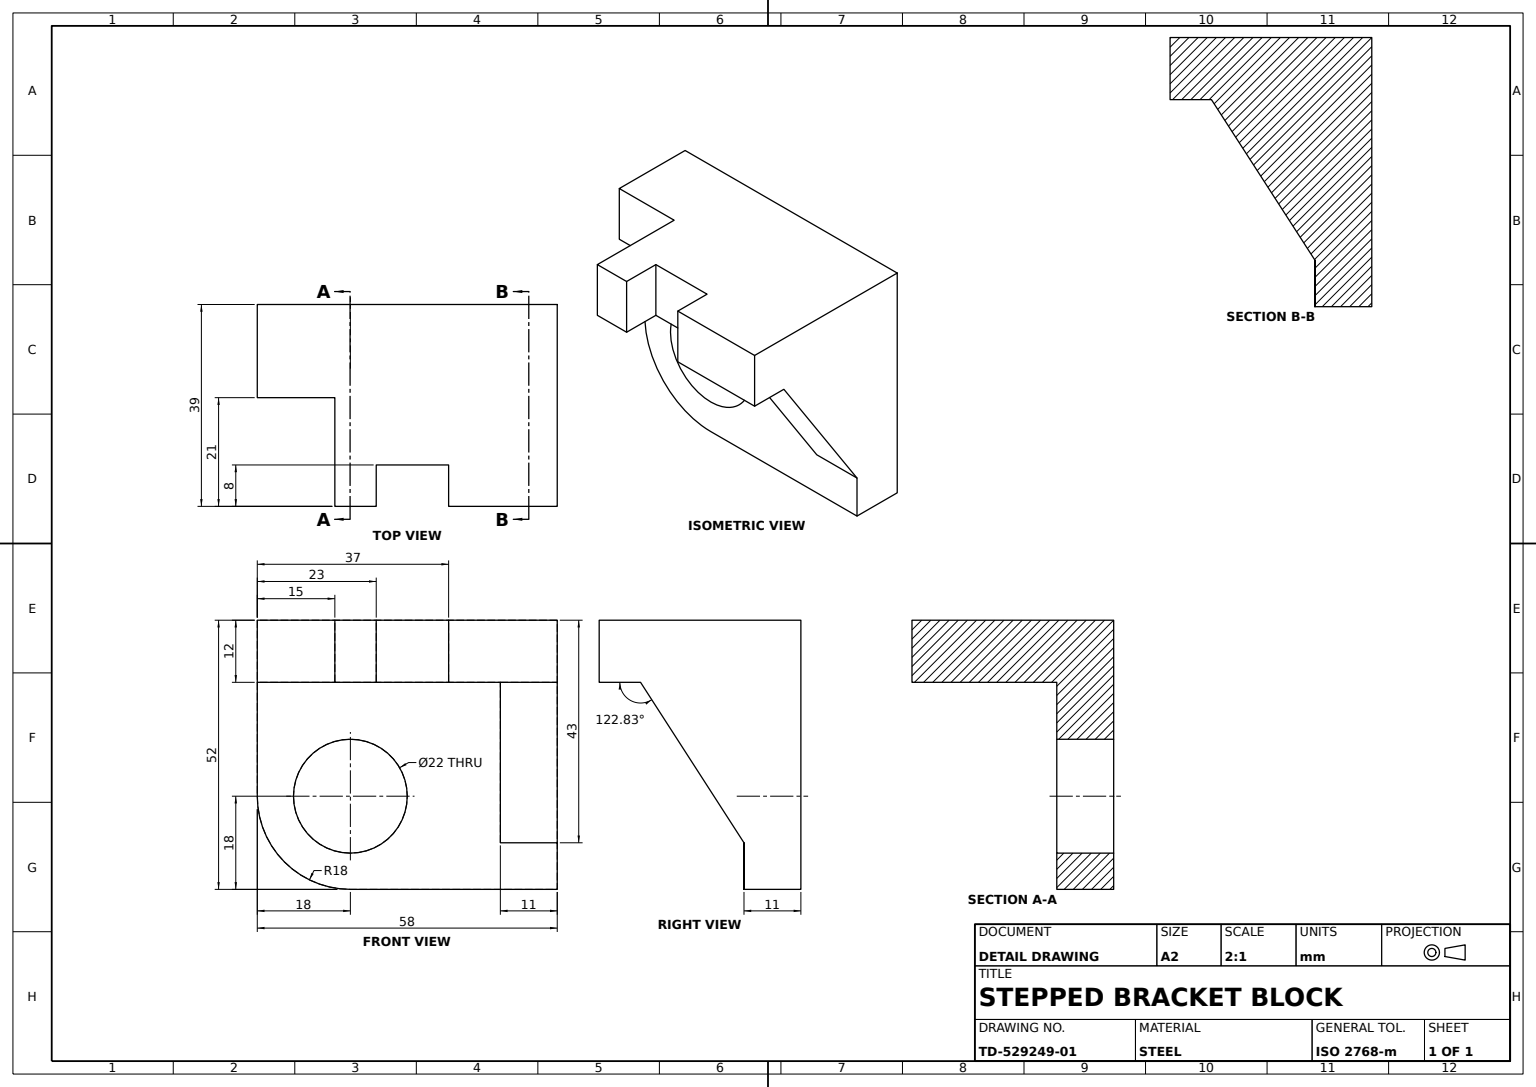
from build123d import *

# Parameters (mm, degrees)
BASE_BLOCK_DEPTH = 11
TOP_PLATE_DEPTH  = 12
GUSSET_RIB_DEPTH = 11
CUT_22_PROFILE_R = 11
CUT_22_DEPTH     = 11


with BuildPart() as part:
    # Base Block Profile → Base Block (new body)
    with BuildSketch(Plane.XY):
        with BuildLine():
            Line((58, 0), (58, -52))
            Line((58, -52), (18, -52))
            ThreePointArc((18, -52), (5.272077939, -46.727922061), (0, -34))
            Line((0, -34), (0, 0))
            Line((0, 0), (58, 0))
        make_face()
    extrude(amount=BASE_BLOCK_DEPTH)

    # Top Plate Profile → Top Plate (add)
    with BuildSketch(Plane(origin=(0, 0, 0), x_dir=(1, 0, 0), z_dir=(0, 1, 0))):
        Polygon((58, -11), (58, -39), (37, -39), (37, -31), (23, -31), (23, -39), (15, -39), (15, -18), (0, -18), (0, -11), align=None)
    extrude(amount=-TOP_PLATE_DEPTH)

    # Gusset Profile → Gusset Rib (add)
    with BuildSketch(Plane(origin=(58, 0, 0), x_dir=(0, 0, -1), z_dir=(1, 0, 0))):
        Polygon((-11, -12), (-31, -12), (-11, -43), align=None)
    extrude(amount=-GUSSET_RIB_DEPTH)

    # Cut Ø22 Profile → Cut Ø22 (cut)
    with BuildSketch(Plane.XY.offset(11)):
        with Locations((18, -34)):
            Circle(CUT_22_PROFILE_R)
    extrude(amount=-CUT_22_DEPTH, mode=Mode.SUBTRACT)


solid = part.part
